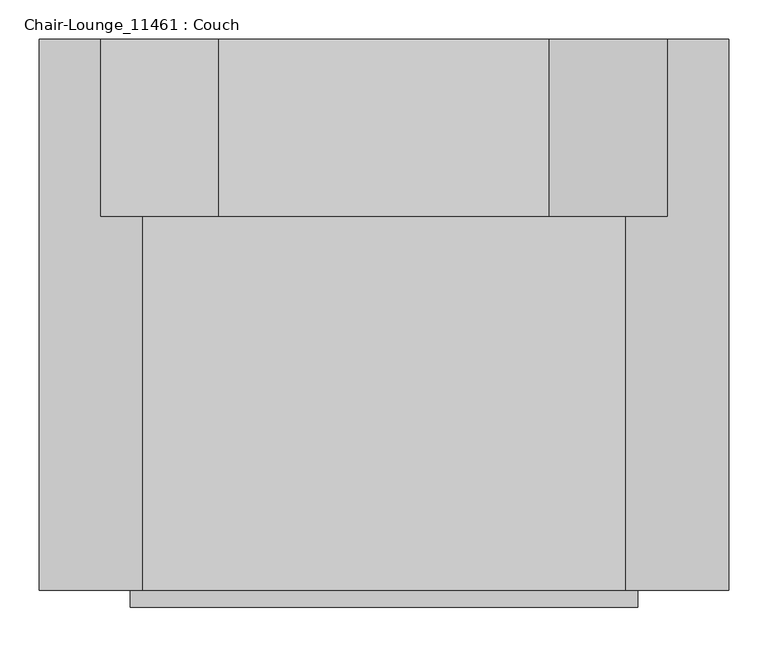
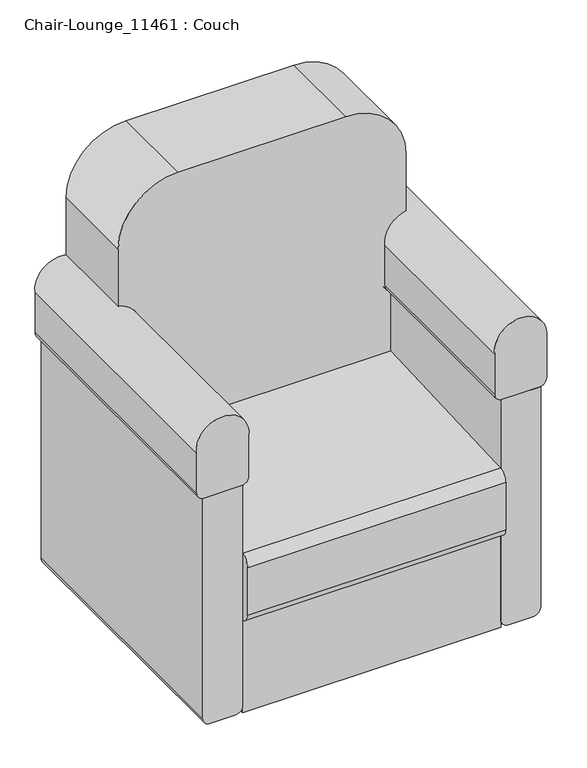
"""IFC4 building model written with IfcOpenShell, lengths in millimetres: furniture geometry, Chair-Lounge_11461 : Couch."""

from ifc_helpers import new_model, si_unit, point, frame, frame_2d, origin, place, context, project, spatial, polyline, circle_curve, trimmed, segment, composite_curve, outline, extrude, source, transform, mapped, element, save
from ifc_brep_helpers import plane_surface, cylinder_surface, revolved_surface, advanced_brep


def chair_lounge_11461_couch_0866092f(model_context):
    return source(origin(), model_context, "Body", "SolidModel", [
        extrude(outline(composite_curve([segment(polyline([(600.6350833, 422.5), (600.6350833, 322.5), (20.0, 322.5)]), True, "CONTINUOUS"), segment(trimmed(circle_curve(frame_2d((20.0, 342.5)), 20.0), [point((20.0, 322.5))], [point((0.0, 342.5))], False, "CARTESIAN"), True, "CONTINUOUS"), segment(polyline([(0.0, 342.5), (0.0, 402.5)]), True, "CONTINUOUS"), segment(trimmed(circle_curve(frame_2d((20.0, 402.5)), 20.0), [point((0.0, 402.5))], [point((20.0, 422.5))], False, "CARTESIAN"), True, "CONTINUOUS"), segment(polyline([(20.0, 422.5), (600.6350833, 422.5)]), True, "CONTINUOUS")], self_intersect=False)), frame((0.0, -700.0, 0.0), z_axis=(0.0, 1.0, 0.0), x_axis=(0.0, 0.0, 1.0)), (0.0, 0.0, 1.0), 700.0),
        extrude(outline(composite_curve([segment(polyline([(600.6350833, -322.5), (600.6350833, -422.5), (20.0, -422.5)]), True, "CONTINUOUS"), segment(trimmed(circle_curve(frame_2d((20.0, -402.5)), 20.0), [point((20.0, -422.5))], [point((0.0, -402.5))], False, "CARTESIAN"), True, "CONTINUOUS"), segment(polyline([(0.0, -402.5), (0.0, -342.5)]), True, "CONTINUOUS"), segment(trimmed(circle_curve(frame_2d((20.0, -342.5)), 20.0), [point((0.0, -342.5))], [point((20.0, -322.5))], False, "CARTESIAN"), True, "CONTINUOUS"), segment(polyline([(20.0, -322.5), (600.6350833, -322.5)]), True, "CONTINUOUS")], self_intersect=False)), frame((0.0, -700.0, 0.0), z_axis=(0.0, 1.0, 0.0), x_axis=(0.0, 0.0, 1.0)), (0.0, 0.0, 1.0), 700.0),
        extrude(outline(composite_curve([segment(polyline([(725.0, -437.5), (620.6350833, -437.5)]), True, "CONTINUOUS"), segment(trimmed(circle_curve(frame_2d((620.6350833, -417.5)), 20.0), [point((620.6350833, -437.5))], [point((600.6350833, -417.5))], False, "CARTESIAN"), True, "CONTINUOUS"), segment(polyline([(600.6350833, -417.5), (600.6350833, -327.5)]), True, "CONTINUOUS"), segment(trimmed(circle_curve(frame_2d((620.6350833, -327.5)), 20.0), [point((600.6350833, -327.5))], [point((620.6350833, -307.5))], False, "CARTESIAN"), True, "CONTINUOUS"), segment(polyline([(620.6350833, -307.5), (725.0, -307.5)]), True, "CONTINUOUS"), segment(trimmed(circle_curve(frame_2d((734.3333333, -372.5)), 65.6666667), [point((725.0, -307.5))], [point((725.0, -437.5))], False, "CARTESIAN"), True, "CONTINUOUS")], self_intersect=False)), frame((0.0, -700.0, 0.0), z_axis=(0.0, 1.0, 0.0), x_axis=(0.0, 0.0, 1.0)), (0.0, 0.0, 1.0), 700.0),
        extrude(outline(composite_curve([segment(polyline([(725.0, 307.5), (620.6350833, 307.5)]), True, "CONTINUOUS"), segment(trimmed(circle_curve(frame_2d((620.6350833, 327.5)), 20.0), [point((620.6350833, 307.5))], [point((600.6350833, 327.5))], False, "CARTESIAN"), True, "CONTINUOUS"), segment(polyline([(600.6350833, 327.5), (600.6350833, 417.5)]), True, "CONTINUOUS"), segment(trimmed(circle_curve(frame_2d((620.6350833, 417.5)), 20.0), [point((600.6350833, 417.5))], [point((620.6350833, 437.5))], False, "CARTESIAN"), True, "CONTINUOUS"), segment(polyline([(620.6350833, 437.5), (725.0, 437.5)]), True, "CONTINUOUS"), segment(trimmed(circle_curve(frame_2d((734.3333333, 372.5)), 65.6666667), [point((725.0, 437.5))], [point((725.0, 307.5))], False, "CARTESIAN"), True, "CONTINUOUS")], self_intersect=False)), frame((0.0, -700.0, 0.0), z_axis=(0.0, 1.0, 0.0), x_axis=(0.0, 0.0, 1.0)), (0.0, 0.0, 1.0), 700.0),
        advanced_brep(
        [(322.5, -225.0, 600.6350833), (307.5, -225.0, 620.0), (307.5, -225.0, 725.0), (360.0, -225.0, 798.799302), (360.0, -225.0, 950.0), (210.0, -225.0, 1100.0), (-210.0, -225.0, 1100.0), (-360.0, -225.0, 950.0), (-360.0, -225.0, 798.799302), (-307.5, -225.0, 725.0), (-307.5, -225.0, 620.0), (-322.5, -225.0, 600.6350833), (-322.5, -225.0, 442.0019827), (322.5, -225.0, 442.0019827), (-322.5, 0.0, 600.6350833), (-307.5, 0.0, 620.0), (-307.5, 0.0, 725.0), (-360.0, 0.0, 798.799302), (-360.0, 0.0, 950.0), (-210.0, 0.0, 1100.0), (210.0, 0.0, 1100.0), (360.0, 0.0, 950.0), (360.0, 0.0, 798.799302), (307.5, 0.0, 725.0), (307.5, 0.0, 620.0), (322.5, 0.0, 600.6350833), (322.5, 0.0, 0.0), (-322.5, 0.0, 0.0), (322.5, -700.0, 420.990686), (322.5, -721.577804, 396.2260222), (322.5, -721.577804, 270.6867304), (322.5, -696.577804, 245.6867304), (322.5, -700.0, 245.6867304), (322.5, -700.0, 0.0), (-322.5, -700.0, 0.0), (-322.5, -700.0, 245.6867304), (-322.5, -696.577804, 245.6867304), (-322.5, -721.577804, 270.6867304), (-322.5, -721.577804, 396.2260222), (-322.5, -700.0, 420.990686)],
        [
            (0, 1, circle_curve(frame((327.5, -225.0, 620.0), z_axis=(0.0, 1.0, 0.0), x_axis=(1.0, 0.0, 0.0)), 20.0)),
            (1, 2),
            (2, 3, circle_curve(frame((372.5, -225.0, 734.3333333), z_axis=(0.0, 1.0, 0.0), x_axis=(1.0, 0.0, 0.0)), 65.6666667)),
            (3, 4),
            (4, 5, circle_curve(frame((210.0, -225.0, 950.0), z_axis=(0.0, -1.0, 0.0), x_axis=(1.0, 0.0, 0.0)), 150.0)),
            (5, 6),
            (6, 7, circle_curve(frame((-210.0, -225.0, 950.0), z_axis=(0.0, -1.0, 0.0), x_axis=(1.0, 0.0, 0.0)), 150.0)),
            (7, 8),
            (8, 9, circle_curve(frame((-372.5, -225.0, 734.3333333), z_axis=(0.0, 1.0, 0.0), x_axis=(1.0, 0.0, 0.0)), 65.6666667)),
            (9, 10),
            (10, 11, circle_curve(frame((-327.5, -225.0, 620.0), z_axis=(0.0, 1.0, 0.0), x_axis=(1.0, 0.0, 0.0)), 20.0)),
            (11, 12),
            (12, 13),
            (13, 0),
            (14, 15, circle_curve(frame((-327.5, 0.0, 620.0), z_axis=(0.0, -1.0, 0.0), x_axis=(1.0, 0.0, 0.0)), 20.0)),
            (15, 16),
            (16, 17, circle_curve(frame((-372.5, 0.0, 734.3333333), z_axis=(0.0, -1.0, 0.0), x_axis=(1.0, 0.0, 0.0)), 65.6666667)),
            (17, 18),
            (18, 19, circle_curve(frame((-210.0, 0.0, 950.0), z_axis=(0.0, 1.0, 0.0), x_axis=(1.0, 0.0, 0.0)), 150.0)),
            (19, 20),
            (20, 21, circle_curve(frame((210.0, 0.0, 950.0), z_axis=(0.0, 1.0, 0.0), x_axis=(1.0, 0.0, 0.0)), 150.0)),
            (21, 22),
            (22, 23, circle_curve(frame((372.5, 0.0, 734.3333333), z_axis=(0.0, -1.0, 0.0), x_axis=(1.0, 0.0, 0.0)), 65.6666667)),
            (23, 24),
            (24, 25, circle_curve(frame((327.5, 0.0, 620.0), z_axis=(0.0, -1.0, 0.0), x_axis=(1.0, 0.0, 0.0)), 20.0)),
            (25, 26),
            (26, 27),
            (27, 14),
            (25, 0),
            (13, 28, circle_curve(frame((322.5, -350.0, -2111.7783973), z_axis=(1.0, 0.0, 0.0), x_axis=(0.0, 1.0, 0.0)), 2556.8377402)),
            (28, 29, circle_curve(frame((322.5, -696.577804, 396.2260222), z_axis=(1.0, 0.0, 0.0), x_axis=(0.0, 1.0, 0.0)), 25.0)),
            (29, 30),
            (30, 31, circle_curve(frame((322.5, -696.577804, 270.6867304), z_axis=(1.0, 0.0, 0.0), x_axis=(0.0, 1.0, 0.0)), 25.0)),
            (31, 32),
            (32, 33),
            (33, 26),
            (24, 1),
            (23, 2),
            (22, 3),
            (21, 4),
            (20, 5),
            (19, 6),
            (18, 7),
            (17, 8),
            (16, 9),
            (15, 10),
            (14, 11),
            (27, 34),
            (34, 35),
            (35, 36),
            (36, 37, circle_curve(frame((-322.5, -696.577804, 270.6867304), z_axis=(-1.0, 0.0, 0.0), x_axis=(0.0, 1.0, 0.0)), 25.0)),
            (37, 38),
            (38, 39, circle_curve(frame((-322.5, -696.577804, 396.2260222), z_axis=(-1.0, 0.0, 0.0), x_axis=(0.0, 1.0, 0.0)), 25.0)),
            (39, 12, circle_curve(frame((-322.5, -350.0, -2111.7783973), z_axis=(-1.0, 0.0, 0.0), x_axis=(0.0, 1.0, 0.0)), 2556.8377402)),
            (39, 28),
            (38, 29),
            (37, 30),
            (36, 31),
            (32, 35),
            (34, 33),
        ],
        [
            plane_surface(frame((322.5, -225.0, 445.0593579), z_axis=(0.0, -1.0, 0.0), x_axis=(0.0, 0.0, 1.0))),
            plane_surface(frame((322.5, 0.0, 445.0593579), z_axis=(0.0, 1.0, 0.0), x_axis=(0.0, 0.0, -1.0))),
            plane_surface(frame((322.5, -225.0, 440.7190596), z_axis=(1.0, 0.0, 0.0), x_axis=(0.0, 1.0, 0.0))),
            revolved_surface(polyline([(347.5, 0.0, 620.0), (347.5, -225.0, 620.0)]), (327.5, 0.0, 620.0), (0.0, 1.0, 0.0)),
            plane_surface(frame((307.5, -225.0, 620.0), z_axis=(1.0, 0.0, 0.0), x_axis=(0.0, 1.0, 0.0))),
            revolved_surface(polyline([(438.1666667, 0.0, 734.3333333), (438.1666667, -225.0, 734.3333333)]), (372.5, 0.0, 734.3333333), (0.0, 1.0, 0.0)),
            plane_surface(frame((360.0, -225.0, 798.799302), z_axis=(1.0, 0.0, 0.0), x_axis=(0.0, 1.0, 0.0))),
            cylinder_surface(frame((210.0, 0.0, 950.0), z_axis=(0.0, -1.0, 0.0), x_axis=(1.0, 0.0, 0.0)), 150.0),
            plane_surface(frame((210.0, -225.0, 1100.0), z_axis=(0.0, 0.0, 1.0), x_axis=(0.0, 1.0, 0.0))),
            cylinder_surface(frame((-210.0, 0.0, 950.0), z_axis=(0.0, -1.0, 0.0), x_axis=(1.0, 0.0, 0.0)), 150.0),
            plane_surface(frame((-360.0, -225.0, 950.0), z_axis=(-1.0, 0.0, 0.0), x_axis=(0.0, 1.0, 0.0))),
            revolved_surface(polyline([(-306.8333333, 0.0, 734.3333333), (-306.8333333, -225.0, 734.3333333)]), (-372.5, 0.0, 734.3333333), (0.0, 1.0, 0.0)),
            plane_surface(frame((-307.5, -225.0, 725.0), z_axis=(-1.0, 0.0, 0.0), x_axis=(0.0, 1.0, 0.0))),
            revolved_surface(polyline([(-307.5, 0.0, 620.0), (-307.5, -225.0, 620.0)]), (-327.5, 0.0, 620.0), (0.0, 1.0, 0.0)),
            plane_surface(frame((-322.5, -225.0, 600.6350833), z_axis=(-1.0, 0.0, 0.0), x_axis=(0.0, 1.0, 0.0))),
            cylinder_surface(frame((-322.5, -350.0, -2111.7783973), z_axis=(1.0, 0.0, 0.0), x_axis=(0.0, 1.0, 0.0)), 2556.8377402),
            cylinder_surface(frame((-322.5, -696.577804, 396.2260222), z_axis=(1.0, 0.0, 0.0), x_axis=(0.0, 1.0, 0.0)), 25.0),
            plane_surface(frame((322.5, -721.577804, 396.2260222), z_axis=(0.0, -1.0, 0.0), x_axis=(-1.0, 0.0, 0.0))),
            cylinder_surface(frame((-322.5, -696.577804, 270.6867304), z_axis=(1.0, 0.0, 0.0), x_axis=(0.0, 1.0, 0.0)), 25.0),
            plane_surface(frame((322.5, -700.0, 245.6867304), z_axis=(0.0, -1.0, 0.0), x_axis=(-1.0, 0.0, 0.0))),
            plane_surface(frame((322.5, -700.0, 0.0), z_axis=(0.0, 0.0, -1.0), x_axis=(-1.0, 0.0, 0.0))),
            plane_surface(frame((322.5, 0.0, 245.6867304), z_axis=(0.0, 0.0, 1.0), x_axis=(-1.0, 0.0, 0.0))),
        ],
        [
            (0, [[1, 2, 3, 4, 5, 6, 7, 8, 9, 10, 11, 12, 13, 14]]),
            (1, [[15, 16, 17, 18, 19, 20, 21, 22, 23, 24, 25, 26, 27, 28]]),
            (2, [[-26, 29, -14, 30, 31, 32, 33, 34, 35, 36]]),
            (3, [[-1, -29, -25, 37]]),
            (4, [[-2, -37, -24, 38]]),
            (5, [[-3, -38, -23, 39]]),
            (6, [[-4, -39, -22, 40]]),
            (7, [[-5, -40, -21, 41]]),
            (8, [[-6, -41, -20, 42]]),
            (9, [[-7, -42, -19, 43]]),
            (10, [[-8, -43, -18, 44]]),
            (11, [[-9, -44, -17, 45]]),
            (12, [[-10, -45, -16, 46]]),
            (13, [[-11, -46, -15, 47]]),
            (14, [[-47, -28, 48, 49, 50, 51, 52, 53, 54, -12]]),
            (15, [[55, -30, -13, -54]]),
            (16, [[-31, -55, -53, 56]]),
            (17, [[-32, -56, -52, 57]]),
            (18, [[-33, -57, -51, 58]]),
            (19, [[-35, 59, -49, 60]]),
            (20, [[-36, -60, -48, -27]]),
            (21, [[-59, -34, -58, -50]]),
        ],
    ),
    ])


if __name__ == "__main__":
    model = new_model("IFC4")
    model_context = context("Model", 3, world=origin())
    ifc_project = project(units=[si_unit("LENGTHUNIT", "METRE", prefix="MILLI")], contexts=[model_context])
    site = spatial("IfcSite", under=ifc_project)
    building = spatial("IfcBuilding", under=site)
    placement = place(None, origin())
    chair_lounge_11461_couch_shape = chair_lounge_11461_couch_0866092f(model_context)
    element("IfcFurniture", 1, ObjectType="Chair-Lounge_11461 : Couch", at=placement, inside=building, context=model_context, shape_type="MappedRepresentation", body=[
        mapped(chair_lounge_11461_couch_shape, transform((0.0, 0.0, 0.0), x_axis=(1.0, 0.0, 0.0), y_axis=(0.0, 1.0, 0.0), z_axis=(0.0, 0.0, 1.0))),
    ])
    save(model, "model.ifc")

# Revit data of these elements
# Type "Chair-Lounge_11461 : Couch"
#   Default Elevation = 0
#   Assembly Code = ""
